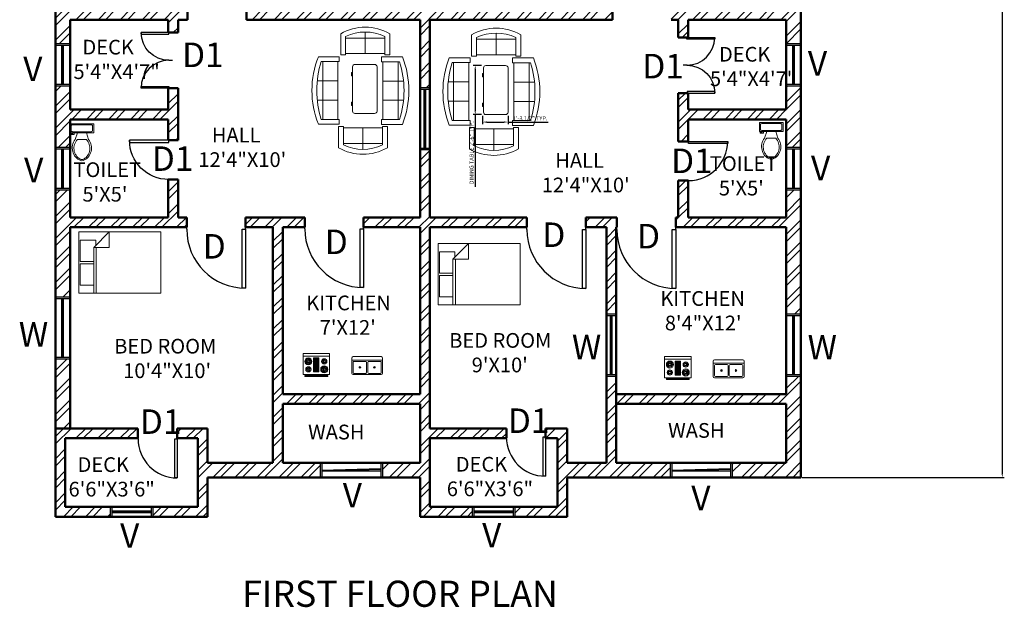
# Model space of a CAD drawing. Units: inches. Extents: x -31438 to -28352, y 12489 to 13610.
# Tile 1 of 5: x -31437 to -30834, y 12489 to 12848. Entities that reach past the tile are written whole.
import ezdxf

# ---------------------------------------------------------------- set-up
doc = ezdxf.new("R2010")
doc.units = ezdxf.units.IN
for name, color, linetype, lineweight in [('A-ANNO-DIMS', 2, 'Continuous', 18), ('A-ANNO-TEXT', 7, 'Continuous', 18), ('A-AREA-IDEN', 3, 'Continuous', 18), ('A-DOOR', 3, 'Continuous', 25), ('A-FLOR-FIXT', 9, 'Continuous', 18), ('A-FURN', 8, 'Continuous', 18), ('A-GLAZ', 4, 'Continuous', 25), ('A-WALL', 7, 'Continuous', 50), ('A-WALL-PATT', 8, 'Continuous', 13)]:
    doc.layers.add(name, color=color, linetype=linetype, lineweight=lineweight)
doc.styles.get("Standard").update_dxf_attribs({"font": 'arial.ttf'})
doc.dimstyles.new('ISO-25', dxfattribs={"dimtxt": 2.5, "dimasz": 2.5, "dimexe": 1.25, "dimexo": 0.625, "dimtad": 1, "dimdec": 0, "dimlunit": 3, "dimtxsty": 'Standard', "dimcen": 2.5, "dimadec": 0, "dimazin": 0, "dimtfac": 1, "dimtdec": 0, "dimtmove": 0, "dimatfit": 3, "dimfxl": 1, "dimarcsym": 0})

# ---------------------------------------------------------------- blocks, each defined once
blk = doc.blocks.new('*U8')
for p, q in [((0, 0), (0, -100)), ((750, 0), (750, -100))]:
    blk.add_line(p, q)
blk.add_lwpolyline([(0, 0), (0, 750), (43.75, 750), (43.75, 0)], close=True)
blk.add_arc((0, 0), 750, 0, 90)
blk = doc.blocks.new('Bed - Queen')
for p, q in [((0, -80.00003), (0, 0)), ((0, 0), (59.99999, 0)), ((59.99999, 0), (59.99999, -80.00003)), ((7.99999, -1.2), (28.79998, -1.2)), ((7.99999, -14.4), (7.99999, -1.2)), ((28.79998, -1.2), (28.79998, -14.4)), ((31.19999, -1.2), (51.99999, -1.2)), ((31.19999, -14.4), (31.19999, -1.2)), ((51.99999, -1.2), (51.99999, -16.4)), ((0, -14.4), (44.8, -14.4)), ((44.8, -16.8), (0, -16.8)), ((59.99999, -29.6), (44.8, -14.4)), ((44.8, -14.4), (44.8, -29.6)), ((51.99999, -16.4), (46.79936, -16.4)), ((44.8, -29.6), (59.99999, -29.6)), ((59.99999, -80.00003), (0, -80.00003))]:
    blk.add_line(p, q)
blk = doc.blocks.new('Range-Oven - 30 in top')
for p, q in [((0, -3), (30, -3)), ((12, -6), (18, -6)), ((13, -20), (13, -6)), ((14, -6), (14, -20)), ((15, -20), (15, -6)), ((16, -6), (16, -20)), ((17, -20), (17, -6)), ((18, -20), (12, -20)), ((6, -24), (6, -25)), ((8, -25), (8, -24)), ((22, -25), (22, -24)), ((24, -24), (24, -25))]:
    blk.add_line(p, q)
for points in [[(0, -24), (0, 0), (30, 0), (30, -24)], [(12, -21), (12, -5), (18, -5), (18, -21)], [(2, -26), (2, -25), (28, -25), (28, -26)]]:
    blk.add_lwpolyline(points, close=True)
for centre, radius in [((6, -9), 4), ((6, -9), 3), ((6, -9), 2), ((6, -9), 1), ((24, -9), 3), ((24, -9), 2), ((24, -9), 1), ((6, -18), 3), ((6, -18), 2), ((6, -18), 1), ((24, -18), 4), ((24, -18), 3), ((24, -18), 2), ((24, -18), 1)]:
    blk.add_circle(centre, radius)
blk = doc.blocks.new('Sink-double - 36 in top')
for p, q in [((-18, -4), (18, -4)), ((-0.75, -18.5), (-0.75, -6.5)), ((0.75, -6.5), (0.75, -18.5))]:
    blk.add_line(p, q)
for points in [[(-16.5, 0), (16.5, 0)], [(-18, -19.5), (-18, -1.5)], [(-16.5, -18.5), (-16.5, -6.5)], [(-15.5, -5.5), (-1.75, -5.5)], [(1.75, -5.5), (15.5, -5.5)], [(16.5, -6.5), (16.5, -18.5)], [(18, -1.5), (18, -19.5)], [(16.5, -21), (-16.5, -21)], [(-1.75, -19.5), (-15.5, -19.5)], [(15.5, -19.5), (1.75, -19.5)]]:
    blk.add_lwpolyline(points)
for centre, radius in [((-8.5, -12.5), 1), ((-8.5, -12.5), 0.5), ((8.5, -12.5), 1), ((8.5, -12.5), 0.5)]:
    blk.add_circle(centre, radius)
for centre, radius, start, end in [((-16.5, -1.5), 1.5, 90, 180), ((16.5, -1.5), 1.5, 0, 90), ((-15.5, -6.5), 1, 90, 180), ((-1.75, -6.5), 1, 0, 90), ((1.75, -6.5), 1, 90, 180), ((15.5, -6.5), 1, 0, 90), ((-16.5, -19.5), 1.5, 180, 270), ((-15.5, -18.5), 1, 180, 270), ((-1.75, -18.5), 1, 270, 0), ((1.75, -18.5), 1, 180, 270), ((15.5, -18.5), 1, 270, 0), ((16.5, -19.5), 1.5, 270, 0)]:
    blk.add_arc(centre, radius, start, end)
blk = doc.blocks.new('Desk - 30 x 60 in.')
for p, q in [((-26.999995, 0), (26.999995, 0)), ((-29.999995, -27), (-29.999995, -3)), ((29.999995, -3), (29.999995, -27)), ((26.999995, -30), (-26.999995, -30)), ((-20.000005, -30), (-20.000005, -31)), ((-20.000005, -31), (-16.000005, -31)), ((-16.000005, -31), (-16.000005, -30)), ((15.999995, -31), (15.999995, -30)), ((19.999995, -31), (15.999995, -31)), ((19.999995, -30), (19.999995, -31))]:
    blk.add_line(p, q)
for centre, start, end in [((-26.499995, -3.5), 98.1301, 171.8699), ((26.499995, -3.5), 8.130102, 81.8699), ((-26.499995, -26.5), 188.1301, 261.8699), ((26.499995, -26.5), 278.1301, 351.8699)]:
    blk.add_arc(centre, 3.535534, start, end)
blk = doc.blocks.new('Sofa - Roundback 7 ft.')
for p, q in [((-36.000027, -34), (-36.000027, -11.4696)), ((-12.00002, -32.4421), (-12.00003, -6.5971)), ((11.99997, -32.4421), (11.99998, -6.5971)), ((35.99998, -34), (35.99998, -11.4696)), ((-35.999844, -13.3819), (35.9998, -13.3819)), ((-36.000027, -32.4421), (35.99998, -32.4421))]:
    blk.add_line(p, q)
for points in [[(-36.000027, -34), (-42.000027, -34), (-42.000027, -8)], [(41.99998, -8), (41.99998, -34), (35.99998, -34)]]:
    blk.add_lwpolyline(points)
for centre, radius, start, end in [((0, -114.25), 114.25, 68.43141, 111.5686), ((-0.00001, -127.1968), 121.1968, 72.72033, 107.2797)]:
    blk.add_arc(centre, radius, start, end)
blk = doc.blocks.new('Sofa - Roundback Loveseat 5 ft.')
for p, q in [((-24, -33.99998), (-24, -11.46958)), ((0, -32.44198), (0, -5.99998)), ((24.00004, -33.99998), (24.00004, -11.46958)), ((-23.9998, -13.38178), (23.99986, -13.38178)), ((-24, -32.44198), (24.00004, -32.44198))]:
    blk.add_line(p, q)
for points in [[(-24, -33.99998), (-30, -33.99998), (-30, -7.99998)], [(30.00004, -7.99998), (30.00004, -33.99998), (24.00004, -33.99998)]]:
    blk.add_lwpolyline(points)
for centre, radius, start, end in [((0, -60.24998), 60.24998, 60.13715, 119.8628), ((0, -61.38438), 55.38444, 64.32083, 115.6792)]:
    blk.add_arc(centre, radius, start, end)
blk = doc.blocks.new('Toilet - top')
for p, q in [((-10, -8.5), (-8, -8.5)), ((-10, -9.5), (-10, -8.5)), ((-8, -8.5), (-8, -8)), ((-7, -8), (-7, -9.5)), ((-4, -8), (-6, -14)), ((4, -8), (6, -14)), ((9.5, -6), (9.5, -2)), ((-7, -9.5), (-10, -9.5)), ((4, -14), (-4, -14))]:
    blk.add_line(p, q)
blk.add_lwpolyline([(10.5, -8), (10.5, 0), (-10.5, 0), (-10.5, -8)], close=True)
for points in [[(-9.5, -2), (-9.5, -6)], [(8.5, -1), (-8.5, -1)], [(-8.5, -7), (8.5, -7)]]:
    blk.add_lwpolyline(points)
for centre, radius, start, end in [((-8.62, -1.88), 0.884, 81.8699, 188.1301), ((-8.62, -6.12), 0.884, 171.8699, 278.1301), ((8.62, -1.88), 0.884, 351.8699, 98.1301), ((8.62, -6.12), 0.884, 261.8699, 8.1301), ((3.52, -21.58), 12.17, 141.46911, 247.97143), ((4.2, -21.82), 11.33, 136.36773, 238.94682), ((-3.52, -21.58), 12.17, 292.02843, 38.53071), ((-4.2, -21.82), 11.33, 301.05301, 43.63209), ((0, -27.88), 4, 245.73182, 294.26817), ((0, -29), 4, 254.86053, 285.13947)]:
    blk.add_arc(centre, radius, start, end)
blk = doc.blocks.new('*D171')
at = {"layer": 'A-ANNO-DIMS', "color": 0, "lineweight": -2, "transparency": 16777216}
for p, q in [((-30958.23, 13407.92), (-30834.47, 13407.92)), ((-30835.72, 13405.42), (-30835.72, 12570.42)), ((-30958.23, 12567.92), (-30834.47, 12567.92))]:
    blk.add_line(p, q, dxfattribs=at)
at = {"layer": 'A-ANNO-DIMS', "color": 0, "transparency": 16777216}
for points in [[(-30836.13, 13405.42), (-30835.3, 13405.42), (-30835.72, 13407.92)], [(-30836.13, 12570.42), (-30835.3, 12570.42), (-30835.72, 12567.92)]]:
    blk.add_solid(points, dxfattribs=at)
at = {"layer": 'Defpoints', "color": 0, "transparency": 16777216}
for p in [(-30958.86, 13407.92), (-30958.86, 12567.92), (-30835.72, 12567.92)]:
    blk.add_point(p, dxfattribs=at)
at = {"layer": 'A-ANNO-DIMS', "color": 0, "transparency": 16777216, "insert": (-30844.51, 12987.92), "char_height": 2.5, "attachment_point": 5, "rotation": 90}
blk.add_mtext("{\\H6.4x;70'}", dxfattribs=at)
blk = doc.blocks.new('WIN-24')
for p, q in [((0, 0), (0, 24)), ((0.5, 0), (0.5, 24))]:
    blk.add_line(p, q)
blk = doc.blocks.new('WIN-36')
for p, q in [((0, 0), (0, 36)), ((0.5, 0), (0.5, 36))]:
    blk.add_line(p, q)
blk = doc.blocks.new('*D201')
at = {"layer": 'A-ANNO-DIMS', "color": 0, "lineweight": -2, "transparency": 16777216}
for p, q in [((-31154.2, 12819.95), (-31159.34, 12819.95)), ((-31158.09, 12817.45), (-31158.09, 12792.33)), ((-31154.2, 12789.83), (-31159.34, 12789.83)), ((-31158.09, 12789.83), (-31158.09, 12745.74))]:
    blk.add_line(p, q, dxfattribs=at)
at = {"layer": 'A-ANNO-DIMS', "color": 0, "transparency": 16777216}
for points in [[(-31158.51, 12817.45), (-31157.67, 12817.45), (-31158.09, 12819.95)], [(-31158.51, 12792.33), (-31157.67, 12792.33), (-31158.09, 12789.83)]]:
    blk.add_solid(points, dxfattribs=at)
at = {"layer": 'Defpoints', "color": 0, "transparency": 16777216}
for p in [(-31153.57, 12819.95), (-31158.09, 12789.83), (-31153.57, 12789.83)]:
    blk.add_point(p, dxfattribs=at)
at = {"layer": 'A-ANNO-DIMS', "color": 0, "transparency": 16777216, "insert": (-31160.01, 12766.53), "char_height": 2.5, "attachment_point": 5, "rotation": 90}
blk.add_mtext('DINING TABLE 2\'-6" TYP.', dxfattribs=at)
blk = doc.blocks.new('*D202')
at = {"layer": 'A-ANNO-DIMS', "color": 0, "lineweight": -2, "transparency": 16777216}
for p, q in [((-31153.57, 12789.2), (-31153.57, 12784.06)), ((-31138.01, 12789.2), (-31138.01, 12784.06)), ((-31151.07, 12785.31), (-31140.51, 12785.31)), ((-31138.01, 12785.31), (-31113.43, 12785.31))]:
    blk.add_line(p, q, dxfattribs=at)
at = {"layer": 'A-ANNO-DIMS', "color": 0, "transparency": 16777216}
for points in [[(-31151.07, 12785.73), (-31151.07, 12784.89), (-31153.57, 12785.31)], [(-31140.51, 12785.73), (-31140.51, 12784.89), (-31138.01, 12785.31)]]:
    blk.add_solid(points, dxfattribs=at)
at = {"layer": 'Defpoints', "color": 0, "transparency": 16777216}
for p in [(-31153.57, 12789.83), (-31138.01, 12789.83), (-31138.01, 12785.31)]:
    blk.add_point(p, dxfattribs=at)
at = {"layer": 'A-ANNO-DIMS', "color": 0, "transparency": 16777216, "insert": (-31124.47, 12787.23), "char_height": 2.5, "attachment_point": 5}
blk.add_mtext('1\'-3 1/2" TYP.', dxfattribs=at)

msp = doc.modelspace()

# ---------------------------------------------------------------- hatches: boundary and pattern name
at = {"layer": 'A-WALL-PATT'}
h = msp.add_hatch(dxfattribs=at)
h.set_pattern_fill('ANSI32', color=256)
h.paths.add_polyline_path([(-30958.86, 13431.92), (-30992.36, 13431.92), (-30992.36, 13425.92), (-30964.86, 13425.92), (-30964.86, 13383.92), (-31006.63, 13383.92), (-31006.63, 13380.92), (-31006.63, 13377.92), (-30958.86, 13377.92)])
h.paths.add_polyline_path([(-30958.86, 13377.92), (-30967.86, 13377.92), (-30967.86, 13330.01), (-30958.86, 13330.01)])
h.paths.add_polyline_path([(-31018.36, 13431.92), (-31051.86, 13431.92), (-31051.86, 13407.92), (-31124.86, 13407.92), (-31124.86, 13398.92), (-31101.86, 13398.92), (-31101.86, 13362.92), (-31185.86, 13362.92), (-31185.86, 13398.92), (-31162.86, 13398.92), (-31162.86, 13407.92), (-31185.86, 13407.92), (-31185.86, 13431.92), (-31217.86, 13431.92), (-31217.86, 13425.92), (-31191.86, 13425.92), (-31191.86, 13383.92), (-31230.51, 13383.92), (-31230.51, 13377.92), (-31191.86, 13377.92), (-31191.86, 13244.1), (-31256.99, 13244.1), (-31256.99, 13238.1), (-31191.86, 13238.1), (-31191.86, 13183.6), (-31185.86, 13183.6), (-31185.86, 13238.1), (-31137.12, 13238.1), (-31137.12, 13244.1), (-31185.86, 13244.1), (-31185.86, 13356.92), (-31101.86, 13356.92), (-31101.86, 13340.51), (-31095.86, 13340.51), (-31095.86, 13398.92), (-31051.86, 13398.92), (-31051.86, 13377.92), (-31030.63, 13377.92), (-31030.63, 13383.92), (-31045.86, 13383.92), (-31045.86, 13425.92), (-31018.36, 13425.92)])
h.paths.add_polyline_path([(-31269.86, 13425.92), (-31243.86, 13425.92), (-31243.86, 13431.92), (-31275.86, 13431.92), (-31275.86, 13407.92), (-31336.86, 13407.92), (-31336.86, 13398.92), (-31305.86, 13398.92), (-31305.86, 13362.92), (-31405.86, 13362.92), (-31405.86, 13398.92), (-31374.86, 13398.92), (-31374.86, 13407.92), (-31414.86, 13407.92), (-31414.86, 13340.51), (-31405.86, 13340.51), (-31405.86, 13356.92), (-31305.86, 13356.92), (-31305.86, 13340.51), (-31299.86, 13340.51), (-31299.86, 13398.92), (-31275.86, 13398.92), (-31275.86, 13377.92), (-31254.51, 13377.92), (-31254.51, 13383.92), (-31269.86, 13383.92)])
h.paths.add_polyline_path([(-31299.86, 13302.51), (-31305.86, 13302.51), (-31305.86, 13244.1), (-31307.44, 13244.1), (-31307.44, 13241.1), (-31307.44, 13238.1), (-31292.99, 13238.1), (-31292.99, 13244.1), (-31299.86, 13244.1)])
h.paths.add_polyline_path([(-31334.44, 13244.1), (-31405.86, 13244.1), (-31405.86, 13302.51), (-31414.86, 13302.51), (-31414.86, 13221.1), (-31405.86, 13221.1), (-31405.86, 13238.1), (-31341.86, 13238.1), (-31341.86, 13213.77), (-31335.86, 13213.77), (-31335.86, 13238.1), (-31334.44, 13238.1)])
h.paths.add_polyline_path([(-31090.53, 13244.1), (-31095.86, 13244.1), (-31095.86, 13302.51), (-31101.86, 13302.51), (-31101.86, 13244.1), (-31113.12, 13244.1), (-31113.12, 13241.1), (-31113.12, 13238.1), (-31090.53, 13238.1)], flags=17)
h.paths.add_polyline_path([(-30958.86, 13292.01), (-30967.86, 13292.01), (-30967.86, 13244.1), (-31033.86, 13244.1), (-31054.53, 13244.1), (-31054.53, 13241.1), (-31054.53, 13238.1), (-31033.86, 13238.1), (-31033.86, 13218.45), (-31027.86, 13218.45), (-31027.86, 13238.1), (-30967.86, 13238.1), (-30967.86, 13221.1), (-30958.86, 13221.1)])
h.paths.add_polyline_path([(-30958.86, 13195.1), (-30967.86, 13195.1), (-30967.86, 13178.1), (-31027.86, 13178.1), (-31027.86, 13194.45), (-31030.86, 13194.45), (-31033.86, 13194.45), (-31033.86, 13162.82), (-31027.86, 13162.82), (-31027.86, 13172.1), (-30967.86, 13172.1), (-30967.86, 13147.51), (-30958.86, 13147.51)])
h.paths.add_polyline_path([(-30958.86, 13121.51), (-30967.86, 13121.51), (-30967.86, 13096.92), (-31027.86, 13096.92), (-31027.86, 13128.82), (-31033.86, 13128.82), (-31033.86, 13096.92), (-31037.31, 13096.92), (-31037.31, 13090.92), (-30967.86, 13090.92), (-30967.86, 13067.92), (-30958.86, 13067.92)])
h.paths.add_polyline_path([(-30958.86, 13029.92), (-30967.86, 13029.92), (-30967.86, 13006.92), (-31025.37, 13006.92), (-31095.86, 13006.92), (-31095.86, 13000.92), (-31081.86, 13000.92), (-31081.86, 12943.92), (-31095.86, 12943.92), (-31095.86, 12937.92), (-31081.86, 12937.92), (-31081.86, 12894.3), (-31075.86, 12894.3), (-31075.86, 13000.92), (-31025.37, 13000.92), (-30967.86, 13000.92), (-30967.86, 12946.42), (-30958.86, 12946.42)])
h.paths.add_polyline_path([(-31121.86, 13006.92), (-31135.86, 13006.92), (-31135.86, 13090.92), (-31081.86, 13090.92), (-31081.86, 13068.53), (-31075.86, 13068.53), (-31075.86, 13090.92), (-31073.31, 13090.92), (-31073.31, 13096.92), (-31141.86, 13096.92), (-31141.86, 13091.1), (-31147.29, 13091.1), (-31147.29, 13085.1), (-31141.86, 13085.1), (-31141.86, 12949.88), (-31146.05, 12949.88), (-31146.05, 12943.88), (-31141.86, 12943.88), (-31141.86, 12853.92), (-31185.86, 12853.92), (-31185.86, 12943.88), (-31182.05, 12943.88), (-31182.05, 12949.88), (-31192.89, 12949.88), (-31192.89, 12943.88), (-31191.86, 12943.88), (-31191.86, 12853.92), (-31231.86, 12853.92), (-31231.86, 12943.88), (-31228.89, 12943.88), (-31228.89, 12949.88), (-31231.86, 12949.88), (-31231.86, 12979.92), (-31272.86, 12979.92), (-31272.86, 12973.92), (-31237.86, 12973.92), (-31237.86, 12853.92), (-31298, 12853.92), (-31298, 12847.92), (-31191.86, 12847.92), (-31191.86, 12806.42), (-31185.86, 12806.42), (-31185.86, 12847.92), (-31074.17, 12847.92), (-31074.17, 12853.92), (-31075.86, 12853.92), (-31075.86, 12870.3), (-31081.86, 12870.3), (-31081.86, 12853.92), (-31135.86, 12853.92), (-31135.86, 12937.92), (-31121.86, 12937.92), (-31121.86, 12943.92), (-31135.86, 12943.92), (-31135.86, 13000.92), (-31121.86, 13000.92)])
h.paths.add_polyline_path([(-30958.86, 12908.42), (-30967.86, 12908.42), (-30967.86, 12853.92), (-31038.17, 12853.92), (-31038.17, 12850.92), (-31038.17, 12847.92), (-31033.86, 12847.92), (-31033.86, 12837.06), (-31027.86, 12837.06), (-31027.86, 12847.92), (-30967.86, 12847.92), (-30967.86, 12833.42), (-30958.86, 12833.42)])
h.paths.add_polyline_path([(-30958.86, 12807.42), (-30967.86, 12807.42), (-30967.86, 12792.92), (-31027.86, 12792.92), (-31027.86, 12803.06), (-31033.86, 12803.06), (-31033.86, 12773.49), (-31027.86, 12773.49), (-31027.86, 12786.92), (-30967.86, 12786.92), (-30967.86, 12769.92), (-30958.86, 12769.92)])
h.paths.add_polyline_path([(-30958.86, 12743.92), (-30967.86, 12743.92), (-30967.86, 12726.92), (-31027.86, 12726.92), (-31027.86, 12749.49), (-31033.86, 12749.49), (-31033.86, 12726.92), (-31035.47, 12726.92), (-31035.47, 12720.92), (-30967.86, 12720.92), (-30967.86, 12667.92), (-30958.86, 12667.92)])
h.paths.add_polyline_path([(-30958.86, 12629.92), (-30967.86, 12629.92), (-30967.86, 12618.92), (-31071.86, 12618.92), (-31071.86, 12612.92), (-30967.86, 12612.92), (-30967.86, 12576.92), (-31000.86, 12576.92), (-31000.86, 12567.92), (-30958.86, 12567.92)])
h.paths.add_polyline_path([(-31038.86, 12576.92), (-31071.86, 12576.92), (-31071.86, 12629.92), (-31077.86, 12629.92), (-31077.86, 12576.92), (-31101.86, 12576.92), (-31101.86, 12597.92), (-31115.03, 12597.92), (-31115.03, 12591.92), (-31107.86, 12591.92), (-31107.86, 12549.92), (-31133.86, 12549.92), (-31133.86, 12543.92), (-31101.86, 12543.92), (-31101.86, 12567.92), (-31038.86, 12567.92)])
h.paths.add_polyline_path([(-31159.86, 12549.92), (-31185.86, 12549.92), (-31185.86, 12591.92), (-31139.03, 12591.92), (-31139.03, 12597.92), (-31185.86, 12597.92), (-31185.86, 12720.92), (-31126.49, 12720.92), (-31126.49, 12726.92), (-31185.86, 12726.92), (-31185.86, 12768.42), (-31191.86, 12768.42), (-31191.86, 12726.92), (-31226.35, 12726.92), (-31226.35, 12720.92), (-31191.86, 12720.92), (-31191.86, 12618.92), (-31275.86, 12618.92), (-31275.86, 12720.92), (-31262.35, 12720.92), (-31262.35, 12726.92), (-31298.57, 12726.92), (-31298.57, 12720.92), (-31281.86, 12720.92), (-31281.86, 12576.92), (-31321.86, 12576.92), (-31321.86, 12597.92), (-31340.38, 12597.92), (-31340.38, 12591.92), (-31327.86, 12591.92), (-31327.86, 12549.92), (-31355.36, 12549.92), (-31355.36, 12543.92), (-31321.86, 12543.92), (-31321.86, 12567.92), (-31252.86, 12567.92), (-31252.86, 12576.92), (-31275.86, 12576.92), (-31275.86, 12612.92), (-31191.86, 12612.92), (-31191.86, 12576.92), (-31214.86, 12576.92), (-31214.86, 12567.92), (-31191.86, 12567.92), (-31191.86, 12543.92), (-31159.86, 12543.92)])
h.paths.add_polyline_path([(-31071.86, 12720.92), (-31071.47, 12726.92), (-31090.49, 12726.92), (-31090.49, 12720.92), (-31077.86, 12720.92), (-31077.86, 12667.92), (-31071.86, 12667.92)])
h.paths.add_polyline_path([(-31381.36, 12549.92), (-31408.86, 12549.92), (-31408.86, 12591.92), (-31364.38, 12591.92), (-31364.38, 12597.92), (-31414.86, 12597.92), (-31414.86, 12543.92), (-31381.36, 12543.92)])
h.paths.add_polyline_path([(-31405.86, 12640.42), (-31414.86, 12640.42), (-31414.86, 12597.92), (-31405.86, 12597.92)])
h.paths.add_polyline_path([(-31405.86, 12720.92), (-31334.57, 12720.92), (-31334.57, 12726.92), (-31339.86, 12726.92), (-31339.86, 12750.16), (-31345.86, 12750.16), (-31345.86, 12726.92), (-31405.86, 12726.92), (-31405.86, 12743.92), (-31414.86, 12743.92), (-31414.86, 12678.42), (-31405.86, 12678.42)])
h.paths.add_polyline_path([(-31339.86, 12806.09), (-31345.86, 12806.09), (-31345.86, 12792.92), (-31405.86, 12792.92), (-31405.86, 12807.42), (-31414.86, 12807.42), (-31414.86, 12769.92), (-31405.86, 12769.92), (-31405.86, 12786.92), (-31345.86, 12786.92), (-31345.86, 12774.16), (-31339.86, 12774.16)])
h.paths.add_polyline_path([(-31334, 12853.92), (-31345.86, 12853.92), (-31345.86, 12973.92), (-31310.86, 12973.92), (-31310.86, 12979.92), (-31405.86, 12979.92), (-31405.86, 13013.51), (-31414.86, 13013.51), (-31414.86, 12971.92), (-31405.86, 12971.92), (-31405.86, 12970.92), (-31409.86, 12970.92), (-31409.86, 12946.92), (-31410.86, 12946.92), (-31410.86, 12970.92), (-31414.86, 12970.92), (-31414.86, 12883.92), (-31405.86, 12883.92), (-31405.86, 12882.92), (-31414.86, 12882.92), (-31414.86, 12833.42), (-31405.86, 12833.42), (-31405.86, 12847.92), (-31345.86, 12847.92), (-31345.86, 12840.09), (-31339.86, 12840.09), (-31339.86, 12847.92), (-31334, 12847.92)])
h.paths.add_polyline_path([(-31351.86, 12937.92), (-31359.89, 12937.92), (-31359.89, 12943.92), (-31351.86, 12943.92), (-31351.86, 12973.92), (-31405.86, 12973.92), (-31405.86, 12943.92), (-31383.89, 12943.92), (-31383.89, 12937.92), (-31405.86, 12937.92), (-31405.86, 12853.92), (-31351.86, 12853.92)], flags=16)
h.paths.add_polyline_path([(-31386.16, 12876.52), (-31390.61, 12876.52), (-31389.24, 12872.41, -0.501323), (-31392.64, 12859.49, -0.132891), (-31394.07, 12859.49, -0.501317), (-31397.46, 12872.41), (-31396.09, 12876.52), (-31398.15, 12876.52), (-31398.15, 12875.49), (-31400.2, 12875.49), (-31400.2, 12876.18), (-31400.22, 12876.52), (-31400.54, 12876.52), (-31400.54, 12882), (-31386.16, 12882)], flags=0)
h.paths.add_polyline_path([(-31387.36, 12877.2), (-31399.17, 12877.2, -0.414214), (-31399.86, 12877.72), (-31399.86, 12880.63, -0.414214), (-31399.35, 12881.31), (-31387.53, 12881.31, -0.414214), (-31386.85, 12880.8), (-31386.85, 12877.89, -0.414214)], flags=0)
h.paths.add_polyline_path([(-31392.23, 12860.41, -0.215004), (-31394.48, 12860.41, -0.48008), (-31396.09, 12872.41), (-31390.61, 12872.41, -0.48008)], flags=0)
h.paths.add_polyline_path([(-31359.87, 12913.86), (-31361.27, 12913.86), (-31361.27, 12937.86), (-31359.87, 12937.86)], flags=0)
h.paths.add_polyline_path([(-31230.55, 13091.1), (-31335.86, 13091.1), (-31335.86, 13129.57), (-31341.86, 13129.57), (-31341.86, 13091.1), (-31405.86, 13091.1), (-31405.86, 13118.6), (-31414.86, 13118.6), (-31414.86, 13051.51), (-31405.86, 13051.51), (-31405.86, 13085.1), (-31230.55, 13085.1)])
h.paths.add_polyline_path([(-31335.86, 13189.77), (-31341.86, 13189.77), (-31341.86, 13178.1), (-31405.86, 13178.1), (-31405.86, 13195.1), (-31414.86, 13195.1), (-31414.86, 13144.6), (-31405.86, 13144.6), (-31405.86, 13172.1), (-31341.86, 13172.1), (-31341.86, 13163.57), (-31335.86, 13163.57)])
h.paths.add_polyline_path([(-31387.11, 12934.37), (-31352.82, 12934.37), (-31352.82, 12965.28), (-31387.11, 12965.28)], flags=8)
h.paths.add_polyline_path([(-31406.38, 12887.22), (-31351.66, 12887.22), (-31351.66, 12920.8), (-31406.38, 12920.8)], flags=24)

# ---------------------------------------------------------------- linework, layer by layer
at = {"layer": 'A-GLAZ'}
for p, q in [((-31414.86, 12833.42), (-31405.86, 12833.42)), ((-31414.86, 12832.42), (-31405.86, 12832.42)), ((-31410.86, 12808.42), (-31410.86, 12832.42)), ((-30967.86, 12833.42), (-30958.86, 12833.42)), ((-30967.86, 12832.42), (-30958.86, 12832.42)), ((-30963.86, 12808.42), (-30963.86, 12832.42)), ((-31414.86, 12808.42), (-31405.86, 12808.42)), ((-31414.86, 12807.42), (-31405.86, 12807.42)), ((-31191.86, 12806.42), (-31185.86, 12806.42)), ((-31191.86, 12805.42), (-31185.86, 12805.42)), ((-31189.36, 12769.42), (-31189.36, 12805.42)), ((-31188.86, 12769.42), (-31188.86, 12805.42)), ((-31188.36, 12769.42), (-31188.36, 12805.42)), ((-30967.86, 12808.42), (-30958.86, 12808.42)), ((-30967.86, 12807.42), (-30958.86, 12807.42)), ((-31414.86, 12769.92), (-31405.86, 12769.92)), ((-31414.86, 12768.92), (-31405.86, 12768.92)), ((-31410.86, 12744.92), (-31410.86, 12768.92)), ((-31191.86, 12769.42), (-31185.86, 12769.42)), ((-31191.86, 12768.42), (-31185.86, 12768.42)), ((-30967.86, 12769.92), (-30958.86, 12769.92)), ((-30967.86, 12768.92), (-30958.86, 12768.92)), ((-30963.86, 12744.92), (-30963.86, 12768.92)), ((-31414.86, 12744.92), (-31405.86, 12744.92)), ((-31414.86, 12743.92), (-31405.86, 12743.92)), ((-30967.86, 12744.92), (-30958.86, 12744.92)), ((-30967.86, 12743.92), (-30958.86, 12743.92)), ((-31414.86, 12678.42), (-31405.86, 12678.42)), ((-31414.86, 12677.42), (-31405.86, 12677.42)), ((-31410.86, 12641.42), (-31410.86, 12677.42)), ((-31077.86, 12667.92), (-31071.86, 12667.92)), ((-31077.86, 12666.92), (-31071.86, 12666.92)), ((-31075.36, 12630.92), (-31075.36, 12666.92)), ((-31074.86, 12630.92), (-31074.86, 12666.92)), ((-31074.36, 12630.92), (-31074.36, 12666.92)), ((-30967.86, 12667.92), (-30958.86, 12667.92)), ((-30967.86, 12666.92), (-30958.86, 12666.92)), ((-30963.86, 12630.92), (-30963.86, 12666.92)), ((-31414.86, 12641.42), (-31405.86, 12641.42)), ((-31414.86, 12640.42), (-31405.86, 12640.42)), ((-31077.86, 12630.92), (-31071.86, 12630.92)), ((-31077.86, 12629.92), (-31071.86, 12629.92)), ((-30967.86, 12630.92), (-30958.86, 12630.92)), ((-30967.86, 12629.92), (-30958.86, 12629.92)), ((-31252.86, 12576.92), (-31252.86, 12567.92)), ((-31251.86, 12576.92), (-31251.86, 12567.92)), ((-31215.86, 12576.92), (-31215.86, 12567.92)), ((-31214.86, 12576.92), (-31214.86, 12567.92)), ((-31038.86, 12576.92), (-31038.86, 12567.92)), ((-31037.86, 12576.92), (-31037.86, 12567.92)), ((-31001.86, 12576.92), (-31001.86, 12567.92)), ((-31000.86, 12576.92), (-31000.86, 12567.92)), ((-31251.86, 12571.92), (-31215.86, 12571.92)), ((-31037.86, 12571.92), (-31001.86, 12571.92)), ((-31381.36, 12549.92), (-31381.36, 12543.92)), ((-31380.36, 12549.92), (-31380.36, 12543.92)), ((-31380.36, 12547.42), (-31356.36, 12547.42)), ((-31380.36, 12546.92), (-31356.36, 12546.92)), ((-31380.36, 12546.42), (-31356.36, 12546.42)), ((-31356.36, 12549.92), (-31356.36, 12543.92)), ((-31355.36, 12549.92), (-31355.36, 12543.92)), ((-31159.86, 12549.92), (-31159.86, 12543.92)), ((-31158.86, 12549.92), (-31158.86, 12543.92)), ((-31158.86, 12547.42), (-31134.86, 12547.42)), ((-31158.86, 12546.92), (-31134.86, 12546.92)), ((-31158.86, 12546.42), (-31134.86, 12546.42)), ((-31134.86, 12549.92), (-31134.86, 12543.92)), ((-31133.86, 12549.92), (-31133.86, 12543.92))]:
    msp.add_line(p, q, dxfattribs=at)
at = {"layer": 'A-WALL'}
for p, q in [((-30958.86, 13431.92), (-30958.86, 12567.92)), ((-31414.86, 12543.92), (-31414.86, 13407.92)), ((-31334, 12853.92), (-31334, 12847.92)), ((-31298, 12853.92), (-31298, 12847.92)), ((-31074.17, 12853.92), (-31074.17, 12847.92)), ((-31405.86, 12792.92), (-31405.86, 12847.92)), ((-31345.86, 12847.92), (-31405.86, 12847.92)), ((-31345.86, 12840.09), (-31345.86, 12847.92)), ((-31345.86, 12840.09), (-31345.86, 12847.92)), ((-31334, 12847.92), (-31339.86, 12847.92)), ((-31339.86, 12840.09), (-31339.86, 12847.92)), ((-31191.86, 12847.92), (-31298, 12847.92)), ((-31191.86, 12726.92), (-31191.86, 12847.92)), ((-31185.86, 12726.92), (-31185.86, 12847.92)), ((-31074.17, 12847.92), (-31185.86, 12847.92)), ((-31033.86, 12847.92), (-31038.17, 12847.92)), ((-31033.86, 12847.92), (-31033.86, 12837.06)), ((-31027.86, 12847.92), (-31027.86, 12837.06)), ((-30967.86, 12847.92), (-31027.86, 12847.92)), ((-30967.86, 12847.92), (-30967.86, 12792.92)), ((-31345.86, 12840.09), (-31339.86, 12840.09)), ((-31033.86, 12837.06), (-31027.86, 12837.06)), ((-31345.86, 12792.92), (-31345.86, 12806.09)), ((-31345.86, 12792.92), (-31345.86, 12806.09)), ((-31345.86, 12806.09), (-31339.86, 12806.09)), ((-31339.86, 12774.16), (-31339.86, 12806.09)), ((-31033.86, 12803.06), (-31027.86, 12803.06)), ((-31033.86, 12803.06), (-31033.86, 12773.49)), ((-31027.86, 12803.06), (-31027.86, 12792.92)), ((-31345.86, 12792.92), (-31405.86, 12792.92)), ((-30967.86, 12792.92), (-31027.86, 12792.92)), ((-31345.86, 12786.92), (-31405.86, 12786.92)), ((-31405.86, 12726.92), (-31405.86, 12786.92)), ((-31345.86, 12774.16), (-31345.86, 12786.92)), ((-31345.86, 12774.16), (-31345.86, 12786.92)), ((-30967.86, 12786.92), (-31027.86, 12786.92)), ((-31027.86, 12786.92), (-31027.86, 12773.49)), ((-30967.86, 12786.92), (-30967.86, 12726.92)), ((-31345.86, 12776.8), (-31345.86, 12776.8)), ((-31345.86, 12774.16), (-31339.86, 12774.16)), ((-31033.86, 12773.49), (-31027.86, 12773.49)), ((-31345.86, 12726.92), (-31345.86, 12750.16)), ((-31345.86, 12726.92), (-31345.86, 12750.16)), ((-31345.86, 12750.16), (-31339.86, 12750.16)), ((-31339.86, 12726.92), (-31339.86, 12750.16)), ((-31033.86, 12749.49), (-31027.86, 12749.49)), ((-31033.86, 12749.49), (-31033.86, 12726.92)), ((-31027.86, 12749.49), (-31027.86, 12726.92)), ((-31345.86, 12726.92), (-31405.86, 12726.92)), ((-31334.57, 12726.92), (-31339.86, 12726.92)), ((-31334.57, 12726.92), (-31334.57, 12720.92)), ((-31298.57, 12726.92), (-31298.57, 12720.92)), ((-31262.35, 12726.92), (-31298.57, 12726.92)), ((-31262.35, 12726.92), (-31262.35, 12720.92)), ((-31191.86, 12726.92), (-31226.35, 12726.92)), ((-31226.35, 12726.92), (-31226.35, 12720.92)), ((-31126.49, 12726.92), (-31185.86, 12726.92)), ((-31126.49, 12726.92), (-31126.49, 12720.92)), ((-31090.49, 12726.92), (-31090.49, 12720.92)), ((-31071.47, 12726.92), (-31090.49, 12726.92)), ((-31071.47, 12720.92), (-31071.47, 12726.92)), ((-31033.86, 12726.92), (-31035.47, 12726.92)), ((-31035.47, 12720.92), (-31035.47, 12726.92)), ((-30967.86, 12726.92), (-31027.86, 12726.92)), ((-31405.86, 12597.92), (-31405.86, 12720.92)), ((-31334.57, 12720.92), (-31405.86, 12720.92)), ((-31281.86, 12720.92), (-31298.57, 12720.92)), ((-31281.86, 12576.92), (-31281.86, 12720.92)), ((-31262.35, 12720.92), (-31275.86, 12720.92)), ((-31275.86, 12618.92), (-31275.86, 12720.92)), ((-31191.86, 12720.92), (-31226.35, 12720.92)), ((-31191.86, 12618.92), (-31191.86, 12720.92)), ((-31185.86, 12597.92), (-31185.86, 12720.92)), ((-31126.49, 12720.92), (-31185.86, 12720.92)), ((-31077.86, 12720.92), (-31090.49, 12720.92)), ((-31077.86, 12576.92), (-31077.86, 12720.92)), ((-31071.86, 12576.92), (-31071.86, 12720.92)), ((-31071.47, 12720.92), (-31071.86, 12720.92)), ((-30967.86, 12720.92), (-31035.47, 12720.92)), ((-30967.86, 12720.92), (-30967.86, 12618.92)), ((-31191.86, 12618.92), (-31275.86, 12618.92)), ((-30967.86, 12618.92), (-31071.86, 12618.92)), ((-31275.86, 12576.92), (-31275.86, 12612.92)), ((-31191.86, 12612.92), (-31275.86, 12612.92)), ((-31191.86, 12576.92), (-31191.86, 12612.92)), ((-30967.86, 12612.92), (-31071.86, 12612.92)), ((-30967.86, 12612.92), (-30967.86, 12576.92)), ((-31364.38, 12597.92), (-31414.86, 12597.92)), ((-31364.38, 12597.92), (-31364.38, 12591.92)), ((-31321.86, 12597.92), (-31340.38, 12597.92)), ((-31340.38, 12597.92), (-31340.38, 12591.92)), ((-31321.86, 12576.92), (-31321.86, 12597.92)), ((-31139.03, 12597.92), (-31185.86, 12597.92)), ((-31139.03, 12597.92), (-31139.03, 12591.92)), ((-31101.86, 12597.92), (-31115.03, 12597.92)), ((-31115.03, 12597.92), (-31115.03, 12591.92)), ((-31101.86, 12576.92), (-31101.86, 12597.92)), ((-31408.86, 12549.92), (-31408.86, 12591.92)), ((-31364.38, 12591.92), (-31408.86, 12591.92)), ((-31327.86, 12591.92), (-31340.38, 12591.92)), ((-31327.86, 12549.92), (-31327.86, 12591.92)), ((-31185.86, 12549.92), (-31185.86, 12591.92)), ((-31139.03, 12591.92), (-31185.86, 12591.92)), ((-31107.86, 12591.92), (-31115.03, 12591.92)), ((-31107.86, 12549.92), (-31107.86, 12591.92)), ((-31281.86, 12576.92), (-31321.86, 12576.92)), ((-31191.86, 12576.92), (-31275.86, 12576.92)), ((-31077.86, 12576.92), (-31101.86, 12576.92)), ((-30967.86, 12576.92), (-31071.86, 12576.92)), ((-31321.86, 12543.92), (-31321.86, 12567.92)), ((-31191.86, 12567.92), (-31321.86, 12567.92)), ((-31191.86, 12543.92), (-31191.86, 12567.92)), ((-30958.86, 12567.92), (-31101.86, 12567.92)), ((-31101.86, 12543.92), (-31101.86, 12567.92)), ((-31327.86, 12549.92), (-31408.86, 12549.92)), ((-31107.86, 12549.92), (-31185.86, 12549.92)), ((-31321.86, 12543.92), (-31414.86, 12543.92)), ((-31321.86, 12543.92), (-31327.86, 12543.92)), ((-31101.86, 12543.92), (-31191.86, 12543.92))]:
    msp.add_line(p, q, dxfattribs=at)

# ---------------------------------------------------------------- block references
at = {"layer": 'A-DOOR'}
for p, xscale, yscale, zscale, rotation in [((-31345.44, 12840.05), -0.022615943267005, 0.022615943267005, 0.022615943267005, 90), ((-31028.59, 12837.03), 0.022615943267005, 0.022615943267005, 0.022615943267005, 270), ((-31345.48, 12806.08), 0.0226814828281586, 0.0226814828281586, 0.0226814828281586, 90), ((-31028.55, 12803.06), -0.0226814828281586, 0.0226814828281586, 0.0226814828281586, 270), ((-31345.57, 12774.14), -0.0319675236688654, 0.0319675236688654, 0.0319675236688654, 90), ((-31027.66, 12773.49), 0.0319999997695785, 0.0319999997695785, 0.0319999997695785, 270), ((-31298.57, 12719.71), 0.0479999999999965, 0.0479999999999965, 0.0479999999999965, 180), ((-31226.35, 12720.07), 0.0479999999999965, 0.0479999999999965, 0.0479999999999965, 180), ((-31090.46, 12719.56), 0.0479999999999965, 0.0479999999999965, 0.0479999999999965, 180), ((-31035.47, 12719.56), 0.0479999999999965, 0.0479999999999965, 0.0479999999999965, 180), ((-31340.35, 12591.65), 0.0320000000000009, 0.0320000000000009, 0.0320000000000009, 180), ((-31115.07, 12592.7), 0.0320000000000009, 0.0320000000000009, 0.0320000000000009, 180)]:
    msp.add_blockref('*U8', p, dxfattribs=dict(at, xscale=xscale, yscale=yscale, zscale=zscale, rotation=rotation))
at = {"layer": 'A-FLOR-FIXT'}
for name, p, xscale, yscale, zscale in [('Toilet - top', (-31398.66, 12784.22), 0.6848978570594845, 0.6848978570594845, 0.6848978570594845), ('Toilet - top', (-30977.02, 12785.03), 0.6848978570594845, 0.6848978570594845, 0.6848978570594845), ('Range-Oven - 30 in top', (-31263.39, 12643.78), 0.5398294676678127, 0.5398294676678127, 0.5398294676678127), ('Sink-double - 36 in top', (-31224.18, 12641.82), 0.5237879159203632, 0.5237879159203632, 0.5237879159203632), ('Range-Oven - 30 in top', (-31042.27, 12641.85), 0.5398294676678127, 0.5398294676678127, 0.5398294676678127), ('Sink-double - 36 in top', (-31003.06, 12639.89), 0.5237879159203632, 0.5237879159203632, 0.5237879159203632)]:
    msp.add_blockref(name, p, dxfattribs=dict(at, xscale=xscale, yscale=yscale, zscale=zscale))
at = {"layer": 'A-FURN', "xscale": 0.4999996666668974, "yscale": 0.4999996666668974, "zscale": 0.4999996666668974}
for p in [(-31225.37, 12843.36), (-31145.27, 12842.7)]:
    msp.add_blockref('Sofa - Roundback Loveseat 5 ft.', p, dxfattribs=at)
at = {"layer": 'A-FURN'}
for name, p, xscale, yscale, zscale, rotation in [('Sofa - Roundback 7 ft.', (-31257.97, 12804.64), 0.4914992872161879, 0.4914992872161879, 0.4914992872161879, 89.99999999999999), ('Sofa - Roundback 7 ft.', (-31198.69, 12804.52), 0.4914992872161879, 0.4914992872161879, 0.4914992872161879, 270), ('Sofa - Roundback 7 ft.', (-31177.86, 12803.99), 0.4914992872161879, 0.4914992872161879, 0.4914992872161879, 89.99999999999999), ('Sofa - Roundback 7 ft.', (-31118.59, 12803.87), 0.4914992872161879, 0.4914992872161879, 0.4914992872161879, 270), ('Desk - 30 x 60 in.', (-31218.11, 12805.54), 0.5020894573147087, 0.5020894573147087, 0.5020894573147087, 270), ('Desk - 30 x 60 in.', (-31138.01, 12804.89), 0.5020894573147087, 0.5020894573147087, 0.5020894573147087, 270), ('Sofa - Roundback Loveseat 5 ft.', (-31226.75, 12765.59), 0.4999996666668974, 0.4999996666668974, 0.4999996666668974, 180), ('Sofa - Roundback Loveseat 5 ft.', (-31146.65, 12764.94), 0.4999996666668974, 0.4999996666668974, 0.4999996666668974, 180), ('Bed - Queen', (-31400.46, 12680.56), 0.6262728017963775, 0.6262728017963775, 0.6262728017963775, 89.99999999999996), ('Bed - Queen', (-31180.77, 12673.43), 0.6262728017963775, 0.6262728017963775, 0.6262728017963775, 89.99999999999996)]:
    msp.add_blockref(name, p, dxfattribs=dict(at, xscale=xscale, yscale=yscale, zscale=zscale, rotation=rotation))
at = {"layer": 'A-GLAZ'}
for name, p in [('WIN-24', (-31410.36, 12808.42)), ('WIN-24', (-30963.36, 12808.42)), ('WIN-24', (-31410.36, 12744.92)), ('WIN-24', (-30963.36, 12744.92)), ('WIN-36', (-31410.36, 12641.42)), ('WIN-36', (-30963.36, 12630.92))]:
    msp.add_blockref(name, p, dxfattribs=at)
at = {"layer": 'A-GLAZ', "rotation": 271.5914471054786}
for p in [(-31251.86, 12572.42), (-31037.86, 12572.42)]:
    msp.add_blockref('WIN-36', p, dxfattribs=at)

# ---------------------------------------------------------------- texts
at = {"layer": 'A-ANNO-TEXT', "attachment_point": 1}
for s, width, insert, char_height in [('{D1}', 148.1867, (-31337.39, 12833.9), 15), ('{V}', 148.1867, (-30954.61, 12828.71), 15), ('{V}', 148.1867, (-31434.57, 12825.35), 15), ('{D1}', 148.1867, (-31055.88, 12827.02), 15), ('{D1}', 148.1867, (-31355.9, 12770.44), 15), ('{D1}', 148.1867, (-31038.29, 12769.08), 15), ('{V}', 148.1867, (-31434.02, 12763.44), 15), ('{V}', 148.1867, (-30952.71, 12764.65), 15), ('{D}', 148.1867, (-31117.05, 12723.88), 15), ('{D}', 148.1867, (-31059.12, 12722.98), 15), ('{D}', 148.1867, (-31324.77, 12716.79), 15), ('{D}', 148.1867, (-31250.11, 12719.52), 15), ('{W}', 148.1867, (-31437.25, 12662.92), 15), ('{W}', 148.1867, (-31098.95, 12655.25), 15), ('{W}', 148.1867, (-30954.79, 12655.09), 15), ('{D1}', 148.1867, (-31363.21, 12609.56), 15), ('{D1}', 148.1867, (-31138.12, 12610.13), 15), ('{V}', 148.1867, (-31239.13, 12564.62), 15), ('{V}', 148.1867, (-31025.96, 12562.9), 15), ('{V}', 148.1867, (-31375.32, 12539.92), 15), ('{V}', 148.1867, (-31153.86, 12540.17), 15), ('{FIRST FLOOR PLAN}', 1791.1862, (-31300.64, 12504.79), 16)]:
    msp.add_mtext_dynamic_manual_height_columns(s, width=width, gutter_width=12.5, heights=[0], dxfattribs=dict(at, insert=insert, char_height=char_height))
at = {"layer": 'A-AREA-IDEN', "char_height": 9, "attachment_point": 1}
for s, insert in [('{  DECK\\P5\'4"X4\'7"}', (-31403.83, 12835.63)), ('{  DECK\\P5\'4"X4\'7"}', (-31014.5, 12831.27)), ('{   HALL\\P12\'4"X10\'}', (-31327.44, 12781.83)), ('{   HALL\\P12\'4"X10\'}', (-31117.38, 12766.32)), ("{TOILET\\P  5'X5'}", (-31014.57, 12764.41)), ("{TOILET\\P  5'X5'}", (-31403.83, 12760.67)), ("{KITCHEN\\P   7'X12'}", (-31261.46, 12679.18)), ('{KITCHEN\\P 8\'4"X12\'}', (-31044.87, 12681.89)), ("{BED ROOM^J     9'X10'}", (-31173.99, 12656.25)), ('{    BED ROOM\\P      10\'4"X10\'}', (-31389.91, 12652.71)), ('{WASH}', (-31260.32, 12600.2)), ('{WASH}', (-31040.11, 12601.19)), ('{  DECK\\P6\'6"X3\'6"}', (-31406.83, 12580.28)), ('{  DECK\\P6\'6"X3\'6"}', (-31175.48, 12580.48))]:
    msp.add_mtext_dynamic_manual_height_columns(s, width=1268.0892, gutter_width=12.5, heights=[0], dxfattribs=dict(at, insert=insert))

# ---------------------------------------------------------------- dimensions: what is measured, and where the dimension line sits
at = {"layer": 'A-ANNO-DIMS'}
for base, p1, p2, angle, text, override, picture, middle in [((-30835.72, 12567.92), (-30958.86, 13407.92), (-30958.86, 12567.92), 90, '{\\H6.4x;<>}', {"dimclrd": 0, "dimclre": 0, "dimclrt": 0}, '*D171', (-30844.51, 12987.92)), ((-31158.09, 12789.83), (-31153.57, 12819.95), (-31153.57, 12789.83), 270, 'DINING TABLE <> TYP.', {"dimdec": 1, "dimlfac": 1, "dimrnd": 0, "dimzin": 1, "dimdsep": 46, "dimlunit": 4, "dimfrac": 2}, '*D201', (-31160.01, 12766.53))]:
    dim = msp.add_linear_dim(base=base, p1=p1, p2=p2, angle=angle, text=text, dimstyle='ISO-25', override=override, dxfattribs=at)
    dim.commit()
    dim.dimension.update_dxf_attribs({"geometry": picture, "text_midpoint": middle})
dim = msp.add_linear_dim(base=(-31138.01, 12785.31), p1=(-31153.57, 12789.83), p2=(-31138.01, 12789.83), text='<> TYP.', dimstyle='ISO-25', override={"dimdec": 1, "dimlfac": 1, "dimrnd": 0, "dimzin": 1, "dimdsep": 46, "dimlunit": 4, "dimfrac": 2}, dxfattribs=at)
dim.commit()
dim.dimension.update_dxf_attribs({"geometry": '*D202', "text_midpoint": (-31124.47, 12787.23)})

doc.saveas('drawing.dxf')
